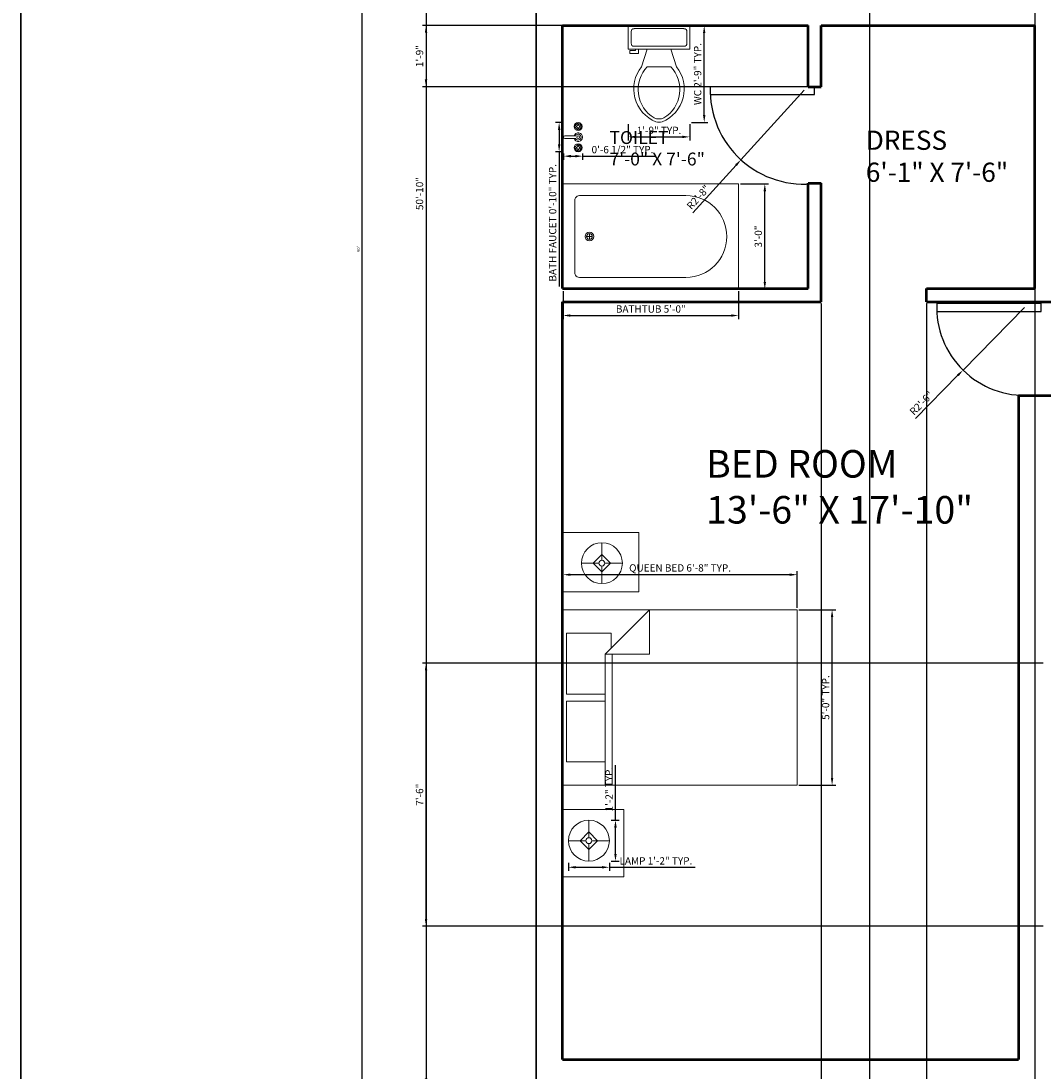
# Model space of a CAD drawing. Units: inches. Extents: x 65 to 818, y -87 to 880.
# Tile 2 of 6: x 65 to 414, y 98 to 457. Entities that reach past the tile are written whole.
import ezdxf

# ---------------------------------------------------------------- set-up
doc = ezdxf.new("R2010")
doc.units = ezdxf.units.IN
for name, color, linetype, lineweight in [('A-ANNO-DIMS', 2, 'Continuous', 18), ('A-ANNO-TTLB', 7, 'Continuous', 35), ('A-AREA-IDEN', 7, 'Continuous', 25), ('A-DOOR', 3, 'Continuous', 25), ('A-FLOR-FIXT', 9, 'Continuous', 18), ('A-FURN', 8, 'Continuous', 18), ('A-WALL', 7, 'Continuous', 50), ('C-PROP', 7, 'Continuous', 35), ('E-LITE', 2, 'Continuous', 18)]:
    doc.layers.add(name, color=color, linetype=linetype, lineweight=lineweight)
doc.styles.get("Standard").update_dxf_attribs({"font": 'arial.ttf'})
doc.dimstyles.new('ISO-25', dxfattribs={"dimtxt": 2.5, "dimasz": 2.5, "dimexe": 1.25, "dimexo": 0.625, "dimtad": 1, "dimtxsty": 'Standard', "dimcen": 2.5, "dimadec": 0, "dimazin": 0, "dimtfac": 1, "dimtmove": 0, "dimatfit": 3, "dimfxl": 1, "dimarcsym": 0})

# ---------------------------------------------------------------- blocks, each defined once
blk = doc.blocks.new('Bed - Queen')
for p, q in [((0, -80.00003), (0, 0)), ((0, 0), (59.99999, 0)), ((59.99999, 0), (59.99999, -80.00003)), ((7.99999, -1.2), (28.79998, -1.2)), ((7.99999, -14.4), (7.99999, -1.2)), ((28.79998, -1.2), (28.79998, -14.4)), ((31.19999, -1.2), (51.99999, -1.2)), ((31.19999, -14.4), (31.19999, -1.2)), ((51.99999, -1.2), (51.99999, -16.4)), ((0, -14.4), (44.8, -14.4)), ((44.8, -16.8), (0, -16.8)), ((59.99999, -29.6), (44.8, -14.4)), ((44.8, -14.4), (44.8, -29.6)), ((51.99999, -16.4), (46.79936, -16.4)), ((44.8, -29.6), (59.99999, -29.6)), ((59.99999, -80.00003), (0, -80.00003))]:
    blk.add_line(p, q)
blk = doc.blocks.new('Toilet - top')
for p, q in [((9.5, -6), (9.5, -2)), ((-10, -8.5), (-8, -8.5)), ((-10, -9.5), (-10, -8.5)), ((-7, -9.5), (-10, -9.5)), ((-8, -8.5), (-8, -8)), ((-7, -8), (-7, -9.5)), ((-4, -8), (-6, -14)), ((4, -8), (6, -14)), ((4, -14), (-4, -14))]:
    blk.add_line(p, q)
blk.add_lwpolyline([(10.5, -8), (10.5, 0), (-10.5, 0), (-10.5, -8)], close=True)
for points in [[(-9.5, -2), (-9.5, -6)], [(8.5, -1), (-8.5, -1)], [(-8.5, -7), (8.5, -7)]]:
    blk.add_lwpolyline(points)
for centre, radius, start, end in [((-8.62, -1.88), 0.884, 81.8699, 188.1301), ((8.62, -1.88), 0.884, 351.8699, 98.1301), ((-8.62, -6.12), 0.884, 171.8699, 278.1301), ((8.62, -6.12), 0.884, 261.8699, 8.1301), ((3.52, -21.58), 12.17, 141.4691, 247.9714), ((4.2, -21.82), 11.33, 136.3677, 238.9468), ((-3.52, -21.58), 12.17, 292.0284, 38.5307), ((-4.2, -21.82), 11.33, 301.053, 43.6321), ((0, -27.88), 4, 245.7318, 294.2682), ((0, -29), 4, 254.8605, 285.1395)]:
    blk.add_arc(centre, radius, start, end)
blk = doc.blocks.new('Bath Tub - 26 x 60 in.')
for p, q in [((9, -17), (9, -19)), ((8, -18), (10, -18))]:
    blk.add_line(p, q)
blk.add_lwpolyline([(0, -36), (0, 0), (60, 0), (60, -36)], close=True)
for points in [[(4, -30), (4, -6)], [(6, -4), (42, -4)], [(42, -32), (6, -32)]]:
    blk.add_lwpolyline(points)
for radius in [1.5, 1]:
    blk.add_circle((9, -18), radius)
for centre, radius, start, end in [((5.75, -5.75), 1.77, 81.8699, 188.1301), ((42, -18), 14, 270, 90), ((5.75, -30.25), 1.77, 171.8699, 278.1301)]:
    blk.add_arc(centre, radius, start, end)
blk = doc.blocks.new('Faucet - Bathroom top')
for p, q in [((-4.107, 0.125), (-4.375, 0.125)), ((-3.75, 0.4788), (-3.75, 0.75)), ((-3.5, 0.482), (-3.5, 0.75)), ((-3.1461, 0.125), (-2.875, 0.125)), ((3.143, 0.125), (2.875, 0.125)), ((3.5, 0.4788), (3.5, 0.75)), ((3.75, 0.482), (3.75, 0.75)), ((4.1039, 0.125), (4.375, 0.125)), ((-4.1039, -0.125), (-4.375, -0.125)), ((-3.75, -0.4821), (-3.75, -0.75)), ((-3.5, -0.4789), (-3.5, -0.75)), ((-3.143, -0.125), (-2.875, -0.125)), ((-0.5, -0.8639), (-0.5, -4.5)), ((0.5, -4.5), (0.5, -0.8631)), ((3.1461, -0.125), (2.875, -0.125)), ((3.5, -0.4821), (3.5, -0.75)), ((3.75, -0.4789), (3.75, -0.75)), ((4.107, -0.125), (4.375, -0.125))]:
    blk.add_line(p, q)
for centre, radius in [((-3.625, 0), 1.375), ((-4.625, 0), 0.2795), ((-3.625, 0), 0.5), ((-3.625, 1), 0.2795), ((-2.625, 0), 0.2795), ((0, 0), 0.5), ((3.625, 0), 1.375), ((2.625, 0), 0.2795), ((3.625, 0), 0.5), ((3.625, 1), 0.2795), ((4.625, 0), 0.2795), ((-3.625, -1), 0.2795), ((3.625, -1), 0.2795)]:
    blk.add_circle(centre, radius)
for centre, radius, start, end in [((-3.625, 0), 1, 105.2407, 164.2093), ((-3.625, 0), 1, 16.44125, 74.07887), ((0, 0), 1.5, 289.6514, 250.3603), ((0, 0), 1, 300.3431, 239.7554), ((3.625, 0), 1, 106.12, 164.0884), ((3.625, 0), 1, 16.23422, 73.90469), ((-3.625, 0), 1, 196.2342, 253.9047), ((-3.625, 0), 1, 286.12, 344.0884), ((3.625, 0), 1, 196.4413, 254.0789), ((3.625, 0), 1, 285.2407, 344.2093), ((0, -4.5), 0.5, 180, 0)]:
    blk.add_arc(centre, radius, start, end)
blk = doc.blocks.new('Lamp - Table')
for p, q in [((0, 7), (0, 1)), ((-1, 0), (-7, 0)), ((0, 3), (-3, 0)), ((-3, 0), (0, -3)), ((3, 0), (0, 3)), ((0, -3), (3, 0)), ((1, 0), (7, 0)), ((0, -1), (0, -7))]:
    blk.add_line(p, q)
for radius in [7, 1]:
    blk.add_circle((0, 0), radius)
blk = doc.blocks.new('*D14')
at = {"layer": 'A-ANNO-DIMS', "color": 0, "lineweight": -2, "transparency": 16777216}
for p, q in [((240.17, 739.04), (179.98, 739.04)), ((181.23, 21.54), (181.23, 736.54)), ((240.17, 19.04), (179.98, 19.04))]:
    blk.add_line(p, q, dxfattribs=at)
at = {"layer": 'A-ANNO-DIMS', "color": 0, "transparency": 16777216}
for points in [[(180.81, 736.54), (181.65, 736.54), (181.23, 739.04)], [(180.81, 21.54), (181.65, 21.54), (181.23, 19.04)]]:
    blk.add_solid(points, dxfattribs=at)
at = {"layer": 'Defpoints', "color": 0, "transparency": 16777216}
for p in [(181.23, 739.04), (240.8, 739.04), (240.8, 19.04)]:
    blk.add_point(p, dxfattribs=at)
at = {"layer": 'A-ANNO-DIMS', "color": 0, "transparency": 16777216, "insert": (180.09, 379.04), "char_height": 1, "attachment_point": 5, "rotation": 90}
blk.add_mtext("60'", dxfattribs=at)
blk = doc.blocks.new('DOOR-LEAF-36-NOM')
blk.add_lwpolyline([(0, 0), (2.67, 0), (2.67, 35.67), (0, 35.67)], close=True)
blk = doc.blocks.new('*D22')
at = {"layer": 'A-ANNO-DIMS', "color": 0, "lineweight": -2, "transparency": 16777216}
for p, q in [((251.8, 169.19), (251.8, 166.46)), ((265.8, 169.19), (265.8, 166.46)), ((254.3, 167.71), (263.3, 167.71)), ((265.8, 167.71), (295.16, 167.71))]:
    blk.add_line(p, q, dxfattribs=at)
at = {"layer": 'A-ANNO-DIMS', "color": 0, "transparency": 16777216}
for points in [[(254.3, 168.13), (254.3, 167.3), (251.8, 167.71)], [(263.3, 168.13), (263.3, 167.3), (265.8, 167.71)]]:
    blk.add_solid(points, dxfattribs=at)
at = {"layer": 'Defpoints', "color": 0, "transparency": 16777216}
for p in [(251.8, 169.81), (265.8, 169.81), (265.8, 167.71)]:
    blk.add_point(p, dxfattribs=at)
at = {"layer": 'A-ANNO-DIMS', "color": 0, "transparency": 16777216, "insert": (281.73, 169.59), "char_height": 2.5, "attachment_point": 5}
blk.add_mtext('LAMP 1\'-2" TYP.', dxfattribs=at)
blk = doc.blocks.new('*D23')
at = {"layer": 'A-ANNO-DIMS', "color": 0, "lineweight": -2, "transparency": 16777216}
for p, q in [((267.9, 183.81), (267.9, 202.57)), ((266.42, 183.81), (269.15, 183.81)), ((267.9, 172.31), (267.9, 181.31)), ((266.42, 169.81), (269.15, 169.81))]:
    blk.add_line(p, q, dxfattribs=at)
at = {"layer": 'A-ANNO-DIMS', "color": 0, "transparency": 16777216}
for points in [[(267.48, 181.31), (268.31, 181.31), (267.9, 183.81)], [(267.48, 172.31), (268.31, 172.31), (267.9, 169.81)]]:
    blk.add_solid(points, dxfattribs=at)
at = {"layer": 'Defpoints', "color": 0, "transparency": 16777216}
for p in [(265.8, 183.81), (267.9, 183.81), (265.8, 169.81)]:
    blk.add_point(p, dxfattribs=at)
at = {"layer": 'A-ANNO-DIMS', "color": 0, "transparency": 16777216, "insert": (266.02, 194.44), "char_height": 2.5, "attachment_point": 5, "rotation": 90}
blk.add_mtext('1\'-2" TYP.', dxfattribs=at)
blk = doc.blocks.new('*D26')
at = {"layer": 'A-ANNO-DIMS', "color": 0, "lineweight": -2, "transparency": 16777216}
for p, q in [((249.99, 256.37), (249.99, 268.99)), ((327.49, 267.74), (252.49, 267.74)), ((329.99, 256.37), (329.99, 268.99))]:
    blk.add_line(p, q, dxfattribs=at)
at = {"layer": 'A-ANNO-DIMS', "color": 0, "transparency": 16777216}
for points in [[(252.49, 268.16), (252.49, 267.32), (249.99, 267.74)], [(327.49, 268.16), (327.49, 267.32), (329.99, 267.74)]]:
    blk.add_solid(points, dxfattribs=at)
at = {"layer": 'Defpoints', "color": 0, "transparency": 16777216}
for p in [(249.99, 267.74), (249.99, 255.74), (329.99, 255.74)]:
    blk.add_point(p, dxfattribs=at)
at = {"layer": 'A-ANNO-DIMS', "color": 0, "transparency": 16777216, "insert": (289.99, 269.73), "char_height": 2.5, "attachment_point": 5}
blk.add_mtext('QUEEN BED 6\'-8" TYP.', dxfattribs=at)
blk = doc.blocks.new('*D27')
at = {"layer": 'A-ANNO-DIMS', "color": 0, "lineweight": -2, "transparency": 16777216}
for p, q in [((330.61, 255.74), (343.24, 255.74)), ((341.99, 198.24), (341.99, 253.24)), ((330.61, 195.74), (343.24, 195.74))]:
    blk.add_line(p, q, dxfattribs=at)
at = {"layer": 'A-ANNO-DIMS', "color": 0, "transparency": 16777216}
for points in [[(341.57, 253.24), (342.4, 253.24), (341.99, 255.74)], [(341.57, 198.24), (342.4, 198.24), (341.99, 195.74)]]:
    blk.add_solid(points, dxfattribs=at)
at = {"layer": 'Defpoints', "color": 0, "transparency": 16777216}
for p in [(329.99, 255.74), (341.99, 255.74), (329.99, 195.74)]:
    blk.add_point(p, dxfattribs=at)
at = {"layer": 'A-ANNO-DIMS', "color": 0, "transparency": 16777216, "insert": (340.09, 225.74), "char_height": 2.5, "attachment_point": 5, "rotation": 90}
blk.add_mtext('5\'-0" TYP.', dxfattribs=at)
blk = doc.blocks.new('*D28')
at = {"layer": 'A-ANNO-DIMS', "color": 0, "lineweight": -2, "transparency": 16777216}
for p, q in [((293.91, 455.41), (299.5, 455.41)), ((298.25, 424.87), (298.25, 452.91)), ((293.91, 422.37), (299.5, 422.37))]:
    blk.add_line(p, q, dxfattribs=at)
at = {"layer": 'A-ANNO-DIMS', "color": 0, "transparency": 16777216}
for points in [[(297.83, 452.91), (298.66, 452.91), (298.25, 455.41)], [(297.83, 424.87), (298.66, 424.87), (298.25, 422.37)]]:
    blk.add_solid(points, dxfattribs=at)
at = {"layer": 'Defpoints', "color": 0, "transparency": 16777216}
for p in [(293.29, 455.41), (298.25, 455.41), (293.29, 422.37)]:
    blk.add_point(p, dxfattribs=at)
at = {"layer": 'A-ANNO-DIMS', "color": 0, "transparency": 16777216, "insert": (296.33, 438.89), "char_height": 2.5, "attachment_point": 5, "rotation": 90}
blk.add_mtext('WC 2\'-9" TYP.', dxfattribs=at)
blk = doc.blocks.new('*D29')
at = {"layer": 'A-ANNO-DIMS', "color": 0, "lineweight": -2, "transparency": 16777216}
for p, q in [((272.29, 421.74), (272.29, 416.16)), ((293.29, 421.74), (293.29, 416.16)), ((274.79, 417.41), (290.79, 417.41))]:
    blk.add_line(p, q, dxfattribs=at)
at = {"layer": 'A-ANNO-DIMS', "color": 0, "transparency": 16777216}
for points in [[(274.79, 417.83), (274.79, 416.99), (272.29, 417.41)], [(290.79, 417.83), (290.79, 416.99), (293.29, 417.41)]]:
    blk.add_solid(points, dxfattribs=at)
at = {"layer": 'Defpoints', "color": 0, "transparency": 16777216}
for p in [(272.29, 422.37), (293.29, 422.37), (293.29, 417.41)]:
    blk.add_point(p, dxfattribs=at)
at = {"layer": 'A-ANNO-DIMS', "color": 0, "transparency": 16777216, "insert": (282.79, 419.31), "char_height": 2.5, "attachment_point": 5}
blk.add_mtext('1\'-9" TYP.', dxfattribs=at)
blk = doc.blocks.new('*D30')
at = {"layer": 'A-ANNO-DIMS', "color": 0, "lineweight": -2, "transparency": 16777216}
for p, q in [((249.98, 364.72), (249.98, 355.1)), ((309.98, 364.72), (309.98, 355.1)), ((252.48, 356.35), (307.48, 356.35))]:
    blk.add_line(p, q, dxfattribs=at)
at = {"layer": 'A-ANNO-DIMS', "color": 0, "transparency": 16777216}
for points in [[(252.48, 356.76), (252.48, 355.93), (249.98, 356.35)], [(307.48, 356.76), (307.48, 355.93), (309.98, 356.35)]]:
    blk.add_solid(points, dxfattribs=at)
at = {"layer": 'Defpoints', "color": 0, "transparency": 16777216}
for p in [(249.98, 365.35), (309.98, 365.35), (309.98, 356.35)]:
    blk.add_point(p, dxfattribs=at)
at = {"layer": 'A-ANNO-DIMS', "color": 0, "transparency": 16777216, "insert": (279.98, 358.25), "char_height": 2.5, "attachment_point": 5}
blk.add_mtext('BATHTUB 5\'-0"', dxfattribs=at)
blk = doc.blocks.new('*D31')
at = {"layer": 'A-ANNO-DIMS', "color": 0, "lineweight": -2, "transparency": 16777216}
for p, q in [((310.61, 401.35), (320.23, 401.35)), ((318.98, 367.85), (318.98, 398.85)), ((310.61, 365.35), (320.23, 365.35))]:
    blk.add_line(p, q, dxfattribs=at)
at = {"layer": 'A-ANNO-DIMS', "color": 0, "transparency": 16777216}
for points in [[(318.56, 398.85), (319.4, 398.85), (318.98, 401.35)], [(318.56, 367.85), (319.4, 367.85), (318.98, 365.35)]]:
    blk.add_solid(points, dxfattribs=at)
at = {"layer": 'Defpoints', "color": 0, "transparency": 16777216}
for p in [(309.98, 401.35), (318.98, 401.35), (309.98, 365.35)]:
    blk.add_point(p, dxfattribs=at)
at = {"layer": 'A-ANNO-DIMS', "color": 0, "transparency": 16777216, "insert": (317.08, 383.35), "char_height": 2.5, "attachment_point": 5, "rotation": 90}
blk.add_mtext('3\'-0"', dxfattribs=at)
blk = doc.blocks.new('*D34')
at = {"layer": 'A-ANNO-DIMS', "color": 0, "lineweight": -2, "transparency": 16777216}
for p, q in [((249.51, 422.32), (247.38, 422.32)), ((248.63, 419.82), (248.63, 414.82)), ((249.51, 412.32), (247.38, 412.32)), ((248.63, 412.32), (248.63, 366.28))]:
    blk.add_line(p, q, dxfattribs=at)
at = {"layer": 'A-ANNO-DIMS', "color": 0, "transparency": 16777216}
for points in [[(248.22, 419.82), (249.05, 419.82), (248.63, 422.32)], [(248.22, 414.82), (249.05, 414.82), (248.63, 412.32)]]:
    blk.add_solid(points, dxfattribs=at)
at = {"layer": 'Defpoints', "color": 0, "transparency": 16777216}
for p in [(250.13, 422.32), (248.63, 412.32), (250.13, 412.32)]:
    blk.add_point(p, dxfattribs=at)
at = {"layer": 'A-ANNO-DIMS', "color": 0, "transparency": 16777216, "insert": (246.72, 388.05), "char_height": 2.5, "attachment_point": 5, "rotation": 90}
blk.add_mtext('BATH FAUCET 0\'-10" TYP.', dxfattribs=at)
blk = doc.blocks.new('*D35')
at = {"layer": 'A-ANNO-DIMS', "color": 0, "lineweight": -2, "transparency": 16777216}
for p, q in [((250.13, 411.7), (250.13, 409.57)), ((252.63, 410.82), (254.13, 410.82)), ((256.63, 411.7), (256.63, 409.57)), ((256.63, 410.82), (281.45, 410.82))]:
    blk.add_line(p, q, dxfattribs=at)
at = {"layer": 'A-ANNO-DIMS', "color": 0, "transparency": 16777216}
for points in [[(252.63, 411.24), (252.63, 410.4), (250.13, 410.82)], [(254.13, 411.24), (254.13, 410.4), (256.63, 410.82)]]:
    blk.add_solid(points, dxfattribs=at)
at = {"layer": 'Defpoints', "color": 0, "transparency": 16777216}
for p in [(250.13, 412.32), (256.63, 412.32), (256.63, 410.82)]:
    blk.add_point(p, dxfattribs=at)
at = {"layer": 'A-ANNO-DIMS', "color": 0, "transparency": 16777216, "insert": (270.29, 412.74), "char_height": 2.5, "attachment_point": 5}
blk.add_mtext('0\'-6 1/2" TYP.', dxfattribs=at)
blk = doc.blocks.new('*D52')
at = {"layer": 'A-ANNO-DIMS', "color": 0, "lineweight": -2, "transparency": 16777216}
for p, q in [((240.17, 703.04), (201.85, 703.04)), ((203.1, 700.54), (203.1, 95.54)), ((249.17, 93.04), (201.85, 93.04))]:
    blk.add_line(p, q, dxfattribs=at)
at = {"layer": 'A-ANNO-DIMS', "color": 0, "transparency": 16777216}
for points in [[(202.68, 700.54), (203.52, 700.54), (203.1, 703.04)], [(202.68, 95.54), (203.52, 95.54), (203.1, 93.04)]]:
    blk.add_solid(points, dxfattribs=at)
at = {"layer": 'Defpoints', "color": 0, "transparency": 16777216}
for p in [(240.8, 703.04), (203.1, 93.04), (249.8, 93.04)]:
    blk.add_point(p, dxfattribs=at)
at = {"layer": 'A-ANNO-DIMS', "color": 0, "transparency": 16777216, "insert": (201.2, 398.04), "char_height": 2.5, "attachment_point": 5, "rotation": 90}
blk.add_mtext('50\'-10"', dxfattribs=at)
blk = doc.blocks.new('*D68')
at = {"layer": 'A-ANNO-DIMS', "color": 0, "lineweight": -2, "transparency": 16777216}
for p, q in [((333.17, 455.54), (201.85, 455.54)), ((203.1, 453.04), (203.1, 437.04)), ((333.17, 434.54), (201.85, 434.54))]:
    blk.add_line(p, q, dxfattribs=at)
at = {"layer": 'A-ANNO-DIMS', "color": 0, "transparency": 16777216}
for points in [[(202.68, 453.04), (203.52, 453.04), (203.1, 455.54)], [(202.68, 437.04), (203.52, 437.04), (203.1, 434.54)]]:
    blk.add_solid(points, dxfattribs=at)
at = {"layer": 'Defpoints', "color": 0, "transparency": 16777216}
for p in [(333.8, 455.54), (203.1, 434.54), (333.8, 434.54)]:
    blk.add_point(p, dxfattribs=at)
at = {"layer": 'A-ANNO-DIMS', "color": 0, "transparency": 16777216, "insert": (201.2, 445.04), "char_height": 2.5, "attachment_point": 5, "rotation": 90}
blk.add_mtext('1\'-9"', dxfattribs=at)
blk = doc.blocks.new('*D72')
at = {"layer": 'A-ANNO-DIMS', "color": 0, "lineweight": -2, "transparency": 16777216}
for p, q in [((354.8, 498.42), (354.8, -19.91)), ((411.3, 498.42), (411.3, -19.91)), ((357.3, -18.66), (408.8, -18.66))]:
    blk.add_line(p, q, dxfattribs=at)
at = {"layer": 'A-ANNO-DIMS', "color": 0, "transparency": 16777216}
for points in [[(357.3, -18.25), (357.3, -19.08), (354.8, -18.66)], [(408.8, -18.25), (408.8, -19.08), (411.3, -18.66)]]:
    blk.add_solid(points, dxfattribs=at)
at = {"layer": 'Defpoints', "color": 0, "transparency": 16777216}
for p in [(354.8, 499.04), (411.3, 499.04), (411.3, -18.66)]:
    blk.add_point(p, dxfattribs=at)
at = {"layer": 'A-ANNO-DIMS', "color": 0, "transparency": 16777216, "insert": (383.05, -16.75), "char_height": 2.5, "attachment_point": 5}
blk.add_mtext('4\'-8 1/2"', dxfattribs=at)
blk = doc.blocks.new('*D73')
at = {"layer": 'A-ANNO-DIMS', "color": 0, "lineweight": -2, "transparency": 16777216}
for p, q in [((338.3, 360.42), (338.3, -19.91)), ((374.3, 360.42), (374.3, -19.91)), ((340.8, -18.66), (371.8, -18.66))]:
    blk.add_line(p, q, dxfattribs=at)
at = {"layer": 'A-ANNO-DIMS', "color": 0, "transparency": 16777216}
for points in [[(340.8, -18.25), (340.8, -19.08), (338.3, -18.66)], [(371.8, -18.25), (371.8, -19.08), (374.3, -18.66)]]:
    blk.add_solid(points, dxfattribs=at)
at = {"layer": 'Defpoints', "color": 0, "transparency": 16777216}
for p in [(338.3, 361.04), (374.3, 361.04), (374.3, -18.66)]:
    blk.add_point(p, dxfattribs=at)
at = {"layer": 'A-ANNO-DIMS', "color": 0, "transparency": 16777216, "insert": (356.3, -16.76), "char_height": 2.5, "attachment_point": 5}
blk.add_mtext('3\'-0"', dxfattribs=at)
blk = doc.blocks.new('*D74')
at = {"layer": 'A-ANNO-DIMS', "color": 0, "lineweight": -2, "transparency": 16777216}
for p, q in [((414.17, 237.54), (201.85, 237.54)), ((203.1, 150.04), (203.1, 235.04)), ((414.17, 147.54), (201.85, 147.54))]:
    blk.add_line(p, q, dxfattribs=at)
at = {"layer": 'A-ANNO-DIMS', "color": 0, "transparency": 16777216}
for points in [[(202.68, 235.04), (203.52, 235.04), (203.1, 237.54)], [(202.68, 150.04), (203.52, 150.04), (203.1, 147.54)]]:
    blk.add_solid(points, dxfattribs=at)
at = {"layer": 'Defpoints', "color": 0, "transparency": 16777216}
for p in [(203.1, 237.54), (414.8, 237.54), (414.8, 147.54)]:
    blk.add_point(p, dxfattribs=at)
at = {"layer": 'A-ANNO-DIMS', "color": 0, "transparency": 16777216, "insert": (201.2, 192.54), "char_height": 2.5, "attachment_point": 5, "rotation": 90}
blk.add_mtext('7\'-6"', dxfattribs=at)
blk = doc.blocks.new('*D80')
at = {"layer": 'A-ANNO-DIMS', "color": 0, "lineweight": -2, "transparency": 16777216}
for p, q in [((332.42, 433.4), (310.82, 409.59)), ((294.4, 391.49), (309.14, 407.74))]:
    blk.add_line(p, q, dxfattribs=at)
at = {"layer": 'A-ANNO-DIMS', "color": 0, "transparency": 16777216}
blk.add_solid([(308.83, 408.02), (309.45, 407.46), (310.82, 409.59)], dxfattribs=at)
at = {"layer": 'Defpoints', "color": 0, "transparency": 16777216}
for p in [(332.42, 433.4), (310.82, 409.59)]:
    blk.add_point(p, dxfattribs=at)
at = {"layer": 'A-ANNO-DIMS', "color": 0, "transparency": 16777216, "insert": (296.45, 396.58), "char_height": 2.5, "attachment_point": 5, "rotation": 47.7824}
blk.add_mtext('R2\'-8"', dxfattribs=at)
blk = doc.blocks.new('*D81')
at = {"layer": 'A-ANNO-DIMS', "color": 0, "lineweight": -2, "transparency": 16777216}
for p, q in [((407.85, 359.13), (386.77, 337.69)), ((370.52, 321.15), (385.02, 335.9))]:
    blk.add_line(p, q, dxfattribs=at)
at = {"layer": 'A-ANNO-DIMS', "color": 0, "transparency": 16777216}
blk.add_solid([(384.72, 336.19), (385.32, 335.61), (386.77, 337.69)], dxfattribs=at)
at = {"layer": 'Defpoints', "color": 0, "transparency": 16777216}
for p in [(407.85, 359.13), (386.77, 337.69)]:
    blk.add_point(p, dxfattribs=at)
at = {"layer": 'A-ANNO-DIMS', "color": 0, "transparency": 16777216, "insert": (372.77, 326.15), "char_height": 2.5, "attachment_point": 5, "rotation": 45.5041}
blk.add_mtext('R2\'-6"', dxfattribs=at)

msp = doc.modelspace()

# ---------------------------------------------------------------- linework, layer by layer
at = {"layer": 'A-ANNO-TTLB'}
msp.add_lwpolyline([(64.55, 880.46), (817.59, 880.46), (817.59, -87.37), (64.55, -87.37)], close=True, dxfattribs=at)
at = {"layer": 'A-DOOR'}
for centre, radius, start, end in [((332.42, 433.4), 32.15, 177.9876, 277.5769), ((407.85, 359.13), 30.07, 177.5374, 273.4708)]:
    msp.add_arc(centre, radius, start, end, dxfattribs=at)
at = {"layer": 'A-FURN'}
for points in [[(249.74, 261.89), (275.86, 261.89), (275.86, 282.18), (249.74, 282.18)], [(249.78, 187.41), (270.79, 187.41), (270.79, 164.42), (249.78, 164.42)]]:
    msp.add_lwpolyline(points, close=True, dxfattribs=at)
at = {"layer": 'A-WALL'}
for p, q in [((249.8, 455.54), (333.8, 455.54)), ((249.8, 365.54), (249.8, 455.54)), ((333.8, 434.54), (333.8, 455.54)), ((338.3, 455.54), (411.3, 455.54)), ((338.3, 434.54), (338.3, 455.54)), ((411.3, 365.54), (411.3, 455.54)), ((333.8, 434.54), (338.3, 434.54)), ((333.8, 365.54), (333.8, 401.54)), ((333.8, 401.54), (338.3, 401.54)), ((338.3, 361.04), (338.3, 401.54)), ((249.8, 365.54), (333.8, 365.54)), ((374.3, 361.04), (374.3, 365.54)), ((374.3, 365.54), (411.3, 365.54)), ((249.8, 361.04), (338.3, 361.04)), ((249.8, 102.04), (249.8, 361.04)), ((374.3, 361.04), (420.3, 361.04)), ((405.8, 329.04), (423.8, 329.04)), ((405.8, 329.04), (405.8, 102.04)), ((249.8, 102.04), (405.8, 102.04))]:
    msp.add_line(p, q, dxfattribs=at)
at = {"layer": 'C-PROP'}
msp.add_line((240.8, 19.04), (240.8, 739.04), dxfattribs=at)

# ---------------------------------------------------------------- block references
at = {"layer": 'A-DOOR'}
for p, rotation in [((335.97, 431.87), 90.00000000000003), ((413.47, 357.76), 89.99999999999984)]:
    msp.add_blockref('DOOR-LEAF-36-NOM', p, dxfattribs=dict(at, rotation=rotation))
at = {"layer": 'A-FLOR-FIXT'}
for name, p in [('Toilet - top', (282.79, 455.41)), ('Bath Tub - 26 x 60 in.', (249.98, 401.35))]:
    msp.add_blockref(name, p, dxfattribs=at)
at = {"layer": 'A-FLOR-FIXT', "rotation": 270}
msp.add_blockref('Faucet - Bathroom top', (255.13, 417.32), dxfattribs=at)
at = {"layer": 'A-FURN', "rotation": 90}
msp.add_blockref('Bed - Queen', (249.99, 195.74), dxfattribs=at)
at = {"layer": 'E-LITE'}
for p in [(263.25, 271.68), (258.8, 176.81)]:
    msp.add_blockref('Lamp - Table', p, dxfattribs=at)

# ---------------------------------------------------------------- texts
at = {"layer": 'A-AREA-IDEN', "attachment_point": 1}
for s, width, gutter_width, insert, char_height in [('TOILET\\P7\'-0" X 7\'-6"', 46.5234, 22.01, (265.84, 419.38), 4.401), ('DRESS\\P6\'-1" X 7\'-6"', 92.0529, 32.82, (353.53, 419.55), 6.5637), ('BED ROOM \\P13\'-6" X 17\'-10"', 167.5252, 47.12, (298.88, 310.35), 9.4236)]:
    msp.add_mtext_dynamic_manual_height_columns(s, width=width, gutter_width=gutter_width, heights=[0], dxfattribs=dict(at, insert=insert, char_height=char_height))

# ---------------------------------------------------------------- dimensions: what is measured, and where the dimension line sits
at = {"layer": 'A-ANNO-DIMS'}
for base, p1, p2, override, picture, middle in [((181.23, 739.04), (240.8, 19.04), (240.8, 739.04), {"dimtxt": 1, "dimdec": 0, "dimlunit": 3, "dimclrd": 0, "dimclre": 0, "dimclrt": 0, "dimtdec": 0}, '*D14', (180.09, 379.04)), ((203.1, 93.04), (240.8, 703.04), (249.8, 93.04), {"dimdec": 1, "dimlfac": 1, "dimrnd": 0, "dimzin": 1, "dimdsep": 46, "dimlunit": 4, "dimfrac": 2}, '*D52', (201.2, 398.04)), ((203.1, 434.54), (333.8, 455.54), (333.8, 434.54), {"dimdec": 1, "dimlfac": 1, "dimrnd": 0, "dimzin": 1, "dimdsep": 46, "dimlunit": 4, "dimfrac": 2}, '*D68', (201.2, 445.04)), ((318.98, 401.35), (309.98, 365.35), (309.98, 401.35), {"dimdec": 1, "dimlfac": 1, "dimrnd": 0, "dimzin": 1, "dimdsep": 46, "dimlunit": 4, "dimfrac": 2}, '*D31', (317.08, 383.35)), ((203.1, 237.54), (414.8, 147.54), (414.8, 237.54), {"dimdec": 1, "dimlfac": 1, "dimrnd": 0, "dimzin": 1, "dimdsep": 46, "dimlunit": 4, "dimfrac": 2}, '*D74', (201.2, 192.54))]:
    dim = msp.add_linear_dim(base=base, p1=p1, p2=p2, angle=90, dimstyle='ISO-25', override=override, dxfattribs=at)
    dim.commit()
    dim.dimension.update_dxf_attribs({"geometry": picture, "text_midpoint": middle})
for base, p1, p2, picture, middle in [((411.3, -18.66), (354.8, 499.04), (411.3, 499.04), '*D72', (383.05, -16.75)), ((374.3, -18.66), (338.3, 361.04), (374.3, 361.04), '*D73', (356.3, -16.76))]:
    dim = msp.add_linear_dim(base=base, p1=p1, p2=p2, dimstyle='ISO-25', override={"dimdec": 1, "dimlfac": 1, "dimrnd": 0, "dimzin": 1, "dimdsep": 46, "dimlunit": 4, "dimfrac": 2}, dxfattribs=at)
    dim.commit()
    dim.dimension.update_dxf_attribs({"geometry": picture, "text_midpoint": middle})
for base, p1, p2, angle, text, picture, middle in [((298.25, 455.41), (293.29, 422.37), (293.29, 455.41), 90, 'WC <> TYP.', '*D28', (296.33, 438.89)), ((248.63, 412.32), (250.13, 422.32), (250.13, 412.32), 270, 'BATH FAUCET <> TYP.', '*D34', (246.72, 388.05)), ((249.99, 267.74), (329.99, 255.74), (249.99, 255.74), 180, 'QUEEN BED <> TYP.', '*D26', (289.99, 269.73)), ((341.99, 255.74), (329.99, 195.74), (329.99, 255.74), 90, '<> TYP.', '*D27', (340.09, 225.74)), ((267.9, 183.81), (265.8, 169.81), (265.8, 183.81), 90, '<> TYP.', '*D23', (266.02, 194.44))]:
    dim = msp.add_linear_dim(base=base, p1=p1, p2=p2, angle=angle, text=text, dimstyle='ISO-25', override={"dimdec": 1, "dimlfac": 1, "dimrnd": 0, "dimzin": 1, "dimdsep": 46, "dimlunit": 4, "dimfrac": 2}, dxfattribs=at)
    dim.commit()
    dim.dimension.update_dxf_attribs({"geometry": picture, "text_midpoint": middle})
for center, mpoint, picture, middle in [((332.423, 433.3971), (310.8196, 409.5865), '*D80', (297.8575, 395.3002)), ((407.85, 359.13), (386.77, 337.69), '*D81', (374.13, 324.82))]:
    dim = msp.add_radius_dim(center=center, mpoint=mpoint, dimstyle='ISO-25', override={"dimdec": 1, "dimlfac": 1, "dimrnd": 0, "dimzin": 1, "dimdsep": 46, "dimlunit": 4, "dimfrac": 2}, dxfattribs=at)
    dim.commit()
    dim.dimension.update_dxf_attribs({"geometry": picture, "text_midpoint": middle, "dimtype": 164})
for base, p1, p2, text, picture, middle in [((293.29, 417.41), (272.29, 422.37), (293.29, 422.37), '<> TYP.', '*D29', (282.79, 419.31)), ((256.63, 410.82), (250.13, 412.32), (256.63, 412.32), '<> TYP.', '*D35', (270.29, 412.74)), ((309.98, 356.35), (249.98, 365.35), (309.98, 365.35), 'BATHTUB <>', '*D30', (279.98, 358.25)), ((265.8, 167.71), (251.8, 169.81), (265.8, 169.81), 'LAMP <> TYP.', '*D22', (281.73, 169.59))]:
    dim = msp.add_linear_dim(base=base, p1=p1, p2=p2, text=text, dimstyle='ISO-25', override={"dimdec": 1, "dimlfac": 1, "dimrnd": 0, "dimzin": 1, "dimdsep": 46, "dimlunit": 4, "dimfrac": 2}, dxfattribs=at)
    dim.commit()
    dim.dimension.update_dxf_attribs({"geometry": picture, "text_midpoint": middle})

doc.saveas('drawing.dxf')
